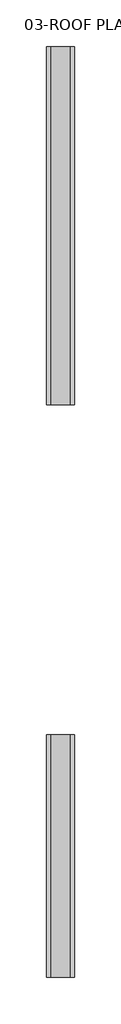
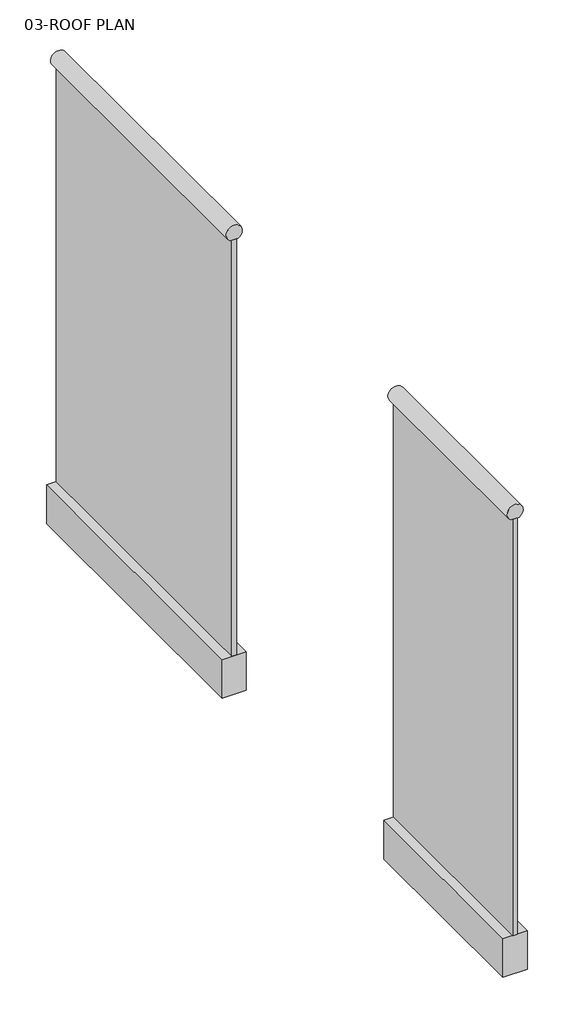
# One storey: 2 railings.
"""IFC4 building model written with IfcOpenShell, lengths in millimetres."""

from ifc_helpers import new_model, si_unit, origin, place, context, project, spatial, transform, mapped, element, save
from components import railing_3627d9a0, railing_ba9b8cd4

model = new_model("IFC4")

# Units and contexts
model_context = context("Model", 3, world=origin())
ifc_project = project(units=[si_unit("LENGTHUNIT", "METRE", prefix="MILLI")], contexts=[model_context])

# Site, building, storey
site = spatial("IfcSite", under=ifc_project)
building = spatial("IfcBuilding", under=site)
storey = spatial("IfcBuildingStorey", under=building, Name="03-ROOF PLAN", Elevation=7350.0)

# Railings
placement = place(None, origin())
railing_shape = railing_3627d9a0(model_context)
element("IfcRailing", 1, at=placement, inside=storey, context=model_context, shape_type="MappedRepresentation", body=[
    mapped(railing_shape, transform((0.0, 0.0, 0.0), x_axis=(1.0, 0.0, 0.0), y_axis=(0.0, 1.0, 0.0), z_axis=(0.0, 0.0, 1.0))),
])
railing_2_shape = railing_ba9b8cd4(model_context)
element("IfcRailing", 2, at=placement, inside=storey, context=model_context, shape_type="MappedRepresentation", body=[
    mapped(railing_2_shape, transform((0.0, 0.0, 0.0), x_axis=(1.0, 0.0, 0.0), y_axis=(0.0, 1.0, 0.0), z_axis=(0.0, 0.0, 1.0))),
])

save(model, "model.ifc")

# Revit data of these elements
# Type
#   Model = "Steel Pro handrail sidebased-LK60/Oak 40/12mm Glass"
#   Manufacturer = "Steelpro"
#   URL = "http://steelpro.bimobject.com/steelpro_lk"
#   Assembly Code = ""
#   built-in parameter 1008619 = -0.082021 (stored number, unit not read)
#   built-in parameter 1008612 = 0.0416667 (stored number, unit not read)
#   built-in parameter 1008611 = 0.0833333 (stored number, unit not read)
#   built-in parameter 1008609 = 4 (stored number, unit not read)
#   built-in parameter 1008604 = 0.166667 (stored number, unit not read)
#   built-in parameter 1008603 = 0.166667 (stored number, unit not read)
#   Railing Height = 1098 mm
#   built-in parameter 1008630 = 2
#   built-in parameter 1008610 = 1
#   built-in parameter 1008605 = 1
# Elements 1, 2 (IfcRailing)
#   Phase Created = New Construction
#   Materials on its faces: "Metal - Aluminum"
# Materials
#   "Metal - Aluminum": colour RGB 247 247 247, transparency 0, Cost = 0
# Room at (-7024.671, 668.593) mm, phase "New Construction", upper level "03-ROOF PLAN", upper offset 4000 mm, lower offset 0 mm
#   Number = "26"
#   Name = "Master Bedroom"
# Room, not placed, phase "New Construction", upper offset 0 mm, lower offset 0 mm
#   Number = "1"
# Room, not placed, phase "New Construction", upper offset 0 mm, lower offset 0 mm
#   Number = "2"
# Room, not placed, phase "New Construction", upper offset 0 mm, lower offset 0 mm
#   Number = "3"
#   Name = "Stairs"
# Room, not placed, phase "New Construction", upper offset 0 mm, lower offset 0 mm
#   Number = "4"
#   Name = "Box room"
# Room at (-3390.544, -6912.295) mm, phase "New Construction", upper level "03-ROOF PLAN", upper offset 4000 mm, lower offset 0 mm
#   Number = "5"
#   Name = "Balcony"
# Room, not placed, phase "New Construction", upper offset 0 mm, lower offset 0 mm
#   Number = "15"
#   Name = "Balcony"
